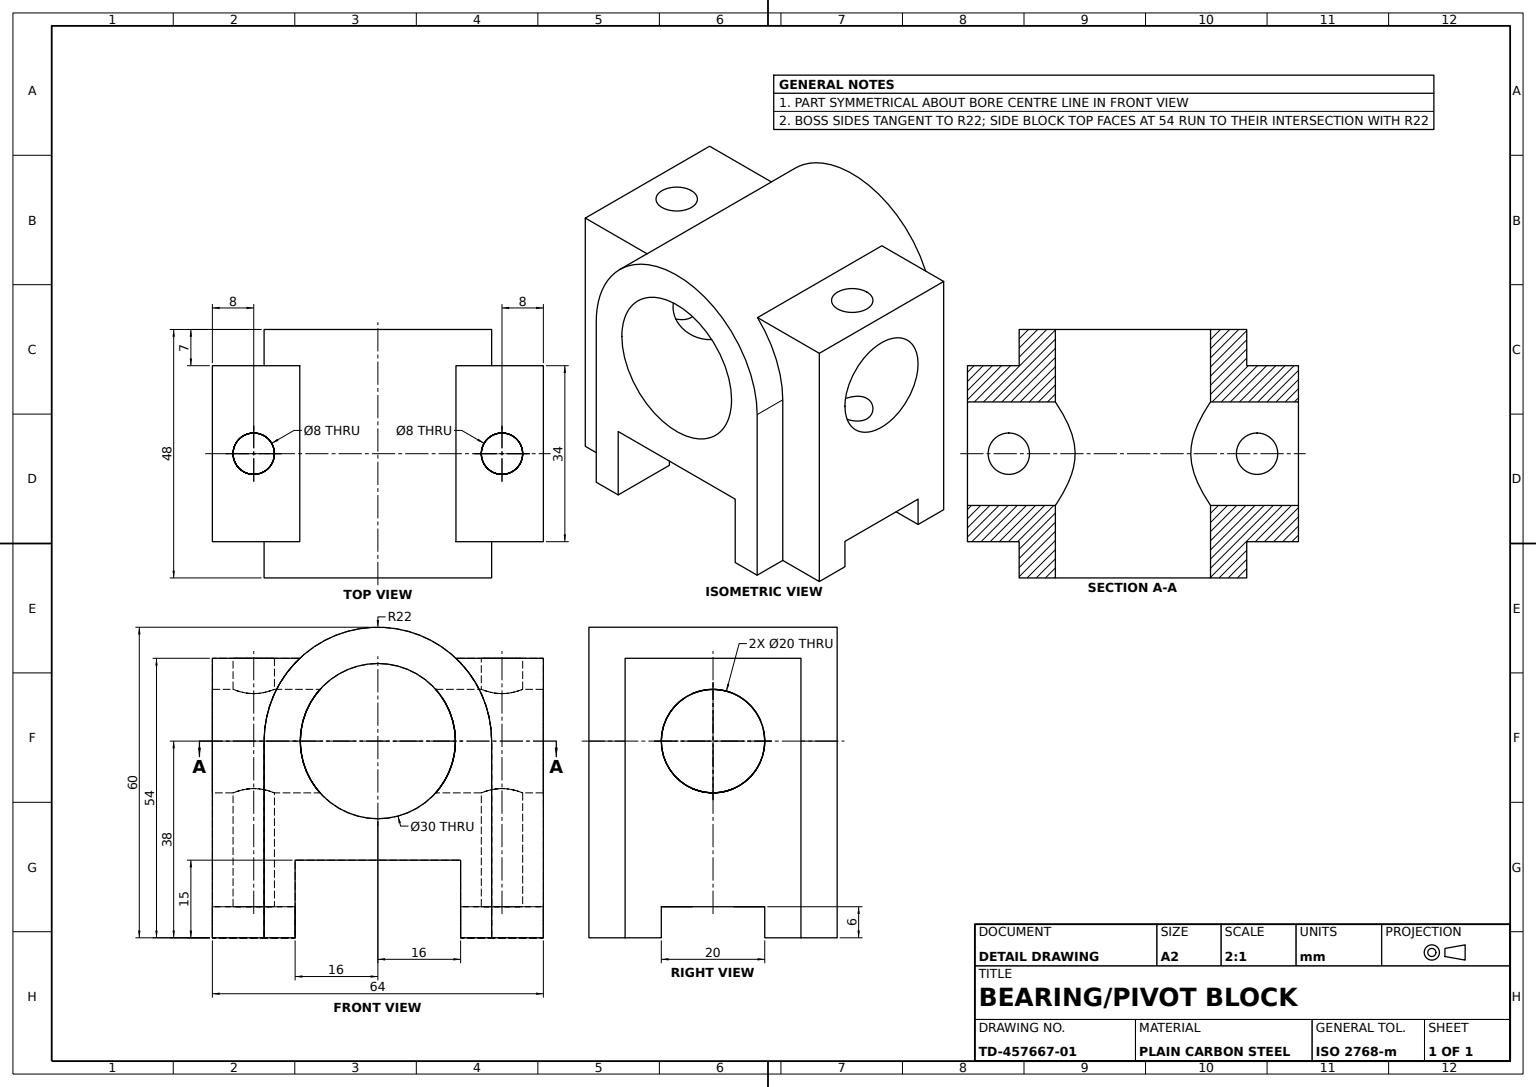
SolidWorks part; units mm, degrees
material "Plain Carbon Steel"
ref_plane "Front Plane" through (0, 0, 0) normal (0, 0, 1) x (1, 0, 0)
ref_plane "Top Plane" through (0, 0, 0) normal (0, 1, 0) x (1, 0, 0)
ref_plane "Right Plane" through (0, 0, 0) normal (1, 0, 0) x (0, 0, -1)
sketch "Base Block Profile" plane through (0, 0, 0) normal (0, 0, 1) x (1, 0, 0)
  line L1 (-32, -27) -> (32, -27)
  line L2 (-32, -27) -> (-32, 27)
  line L3 (-32, 27) -> (32, 27)
  line L4 (32, -27) -> (32, 27)
  line L5 (-32, -27) -> (32, 27) construction
  line L6 (-32, 27) -> (32, -27) construction
  point P0 (0, 0)
  dimension "D1" = 54
  dimension "D2" = 64
extrude "Base Block" add sketch "Base Block Profile" along normal mid plane 34
sketch "Housing Boss Profile" plane through (0, 0, 0) normal (0, 0, 1) x (1, 0, 0)
  line L0 (-32, -27) -> (32, -27) construction
  line L1 (-22, 11) -> (-22, -27)
  line L2 (-22, -27) -> (22, -27)
  line L3 (22, -27) -> (22, 11)
  arc A0 (22, 11) -> (-22, 11) centre (0, 11) ccw
  dimension "D1" = 44
  dimension "D2" = 38
extrude "Bearing Housing Boss" add sketch "Housing Boss Profile" along normal mid plane 48
sketch "Main Bore Profile" plane through (0, 0, 24) normal (0, 0, 1) x (1, 0, 0)
  line L0 (-22, -27) -> (22, -27) construction
  line L1 (-16, -27) -> (16, -27)
  line L2 (-16, -27) -> (-16, -12)
  line L3 (-16, -12) -> (16, -12)
  line L4 (16, -27) -> (16, -12)
  circle A0 centre (0, 11) radius 15
  arc A1 (22, 11) -> (-22, 11) centre (0, 11) ccw construction
  point P14 (0, -12)
  dimension "D1" = 30
  dimension "D2" = 32
  dimension "D3" = 15
extrude "Main Bore" cut sketch "Main Bore Profile" against normal up to surface (48 mm away) up to face at (0, -2.5, -24)
sketch "Cross Hole Profile" plane through (-32, 0, 0) normal (-1, 0, 0) x (0, 0, 1)
  line L0 (17, -27) -> (-17, -27) construction
  line L1 (17, 27) -> (-17, 27) construction
  line L3 (-10, -27) -> (10, -27)
  line L4 (-10, -27) -> (-10, -21)
  line L5 (-10, -21) -> (10, -21)
  line L6 (10, -27) -> (10, -21)
  circle A0 centre (0, 11) radius 10
  point P4 (0, -21)
  point P7 (0, 27)
  dimension "D1" = 20
  dimension "D2" = 38
  dimension "D3" = 20
  dimension "D4" = 6
extrude "Cross Holes" cut sketch "Cross Hole Profile" against normal up to surface (64 mm away) up to face at (32, 0, 0)
sketch "Top Pin Hole Profile" plane through (0, 27, 0) normal (0, 1, 0) x (1, 0, 0)
  line L0 (-36.2162, 0) -> (40.7044, 0) construction
  line L1 (0, 0) -> (0, 20.2659) construction
  circle A0 centre (-24, 0) radius 4
  circle A1 centre (24, 0) radius 4
  dimension "D1" = 8
  dimension "D2" = 48
extrude "Top Pin Holes" cut sketch "Top Pin Hole Profile" against normal up to surface (48 mm away) up to face at (-24, -21, 0)
